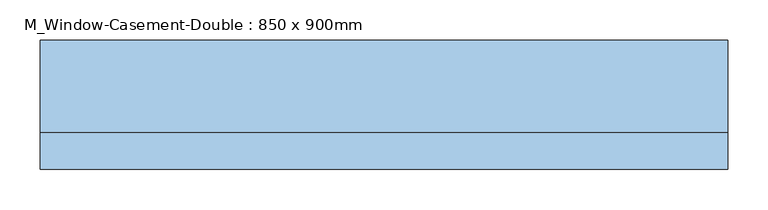
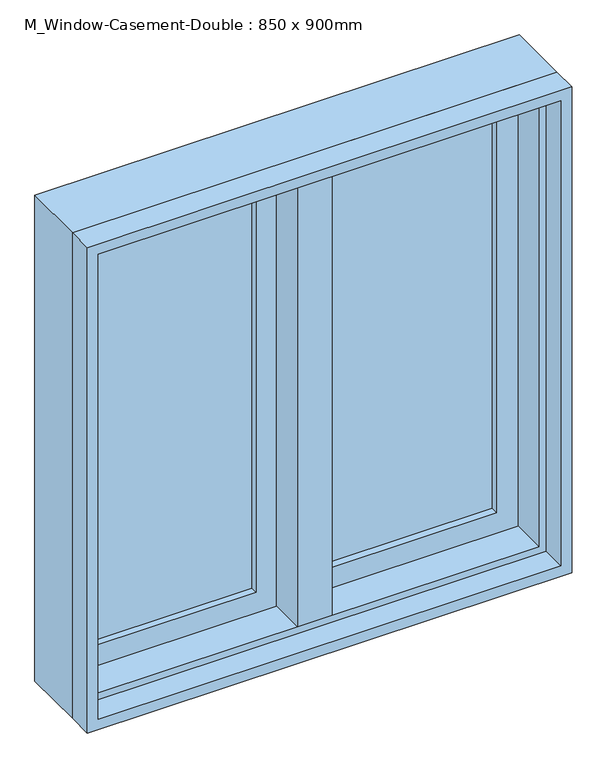
"""IFC4 building model written with IfcOpenShell, lengths in millimetres: window geometry, M_Window-Casement-Double : 850 x 900mm."""

from ifc_helpers import new_model, si_unit, frame, origin, place, context, project, spatial, polyline, outline, extrude, faceted_brep, source, transform, mapped, element, save


def m_window_casement_double_850_x_900mm_77c4388a(model_context):
    return source(origin(), model_context, "Body", "SolidModel", [
        faceted_brep([(9.525, 89.05, 1787.3), (-9.525, 89.05, 1787.3), (-9.525, 38.25, 1787.3), (9.525, 38.25, 1787.3), (9.525, 89.05, 912.7), (9.525, 38.25, 912.7), (-9.525, 38.25, 912.7), (-9.525, 89.05, 912.7), (-9.525, 38.25, 931.75), (-9.525, 38.25, 1768.25), (-30.1625, 38.25, 931.75), (-30.1625, 38.25, 1768.25), (-30.1625, -25.25, 931.75), (-30.1625, -25.25, 1768.25), (30.1625, -25.25, 931.75), (30.1625, -25.25, 1768.25), (30.1625, 38.25, 931.75), (30.1625, 38.25, 1768.25), (9.525, 38.25, 931.75), (9.525, 38.25, 1768.25)], [[[0, 1, 2, 3]], [[4, 5, 6, 7]], [[1, 0, 4, 7]], [[2, 1, 7, 6, 8, 9]], [[9, 8, 10, 11]], [[11, 10, 12, 13]], [[13, 12, 14, 15]], [[15, 14, 16, 17]], [[17, 16, 18, 19]], [[0, 3, 19, 18, 5, 4]], [[18, 8, 6, 5]], [[9, 19, 3, 2]], [[8, 18, 16, 14, 12, 10]], [[19, 9, 11, 13, 15, 17]]]),
        extrude(outline(polyline([(-66.675, 70.0), (-66.675, 63.65), (-355.15, 63.65), (-355.15, 70.0), (-66.675, 70.0)])), frame((0.0, 0.0, 969.85), z_axis=(0.0, 0.0, 1.0), x_axis=(1.0, 0.0, 0.0)), (0.0, 0.0, 1.0), 760.3),
        extrude(outline(polyline([(-355.15, 50.95), (-355.15, 57.3), (-66.675, 57.3), (-66.675, 50.95), (-355.15, 50.95)])), frame((0.0, 0.0, 969.85), z_axis=(0.0, 0.0, 1.0), x_axis=(1.0, 0.0, 0.0)), (0.0, 0.0, 1.0), 760.3),
        extrude(outline(polyline([(355.15, 70.0), (355.15, 63.65), (66.675, 63.65), (66.675, 70.0), (355.15, 70.0)])), frame((0.0, 0.0, 969.85), z_axis=(0.0, 0.0, 1.0), x_axis=(1.0, 0.0, 0.0)), (0.0, 0.0, 1.0), 760.3),
        extrude(outline(polyline([(66.675, 50.95), (66.675, 57.3), (355.15, 57.3), (355.15, 50.95), (66.675, 50.95)])), frame((0.0, 0.0, 969.85), z_axis=(0.0, 0.0, 1.0), x_axis=(1.0, 0.0, 0.0)), (0.0, 0.0, 1.0), 760.3),
        extrude(outline(polyline([(1787.3, -412.3), (912.7, -412.3), (912.7, -9.525), (1787.3, -9.525), (1787.3, -412.3)]), holes=[polyline([(1730.15, -66.675), (969.85, -66.675), (969.85, -355.15), (1730.15, -355.15), (1730.15, -66.675)])]), frame((0.0, 38.25, 0.0), z_axis=(0.0, 1.0, 0.0), x_axis=(0.0, 0.0, 1.0)), (0.0, 0.0, 1.0), 44.45),
        extrude(outline(polyline([(912.7, 412.3), (1787.3, 412.3), (1787.3, 9.525), (912.7, 9.525), (912.7, 412.3)]), holes=[polyline([(969.85, 66.675), (1730.15, 66.675), (1730.15, 355.15), (969.85, 355.15), (969.85, 66.675)])]), frame((0.0, 38.25, 0.0), z_axis=(0.0, 1.0, 0.0), x_axis=(0.0, 0.0, 1.0)), (0.0, 0.0, 1.0), 44.45),
        extrude(outline(polyline([(1800.0, -425.0), (900.0, -425.0), (900.0, 425.0), (1800.0, 425.0), (1800.0, -425.0)]), holes=[polyline([(1780.95, 405.95), (919.05, 405.95), (919.05, -405.95), (1780.95, -405.95), (1780.95, 405.95)])]), frame((0.0, -70.0, 0.0), z_axis=(0.0, 1.0, 0.0), x_axis=(0.0, 0.0, 1.0)), (0.0, 0.0, 1.0), 44.75),
        faceted_brep([(393.25, 38.25, 1768.25), (393.25, -25.25, 1768.25), (-393.25, -25.25, 1768.25), (-393.25, 38.25, 1768.25), (412.3, 89.05, 1787.3), (412.3, 38.25, 1787.3), (-412.3, 38.25, 1787.3), (-412.3, 89.05, 1787.3), (425.0, -25.25, 1800.0), (425.0, 89.05, 1800.0), (-425.0, 89.05, 1800.0), (-425.0, -25.25, 1800.0), (-393.25, -25.25, 931.75), (-393.25, 38.25, 931.75), (-412.3, 38.25, 912.7), (-412.3, 89.05, 912.7), (-425.0, 89.05, 900.0), (-425.0, -25.25, 900.0), (393.25, -25.25, 931.75), (393.25, 38.25, 931.75), (412.3, 38.25, 912.7), (412.3, 89.05, 912.7), (425.0, 89.05, 900.0), (425.0, -25.25, 900.0)], [[[0, 1, 2, 3]], [[4, 5, 6, 7]], [[8, 9, 10, 11]], [[3, 2, 12, 13]], [[7, 6, 14, 15]], [[11, 10, 16, 17]], [[13, 12, 18, 19]], [[15, 14, 20, 21]], [[17, 16, 22, 23]], [[11, 17, 23, 8], [1, 18, 12, 2]], [[19, 18, 1, 0]], [[5, 20, 14, 6], [3, 13, 19, 0]], [[21, 20, 5, 4]], [[23, 22, 9, 8]], [[9, 22, 16, 10], [7, 15, 21, 4]]]),
    ])


if __name__ == "__main__":
    model = new_model("IFC4")
    model_context = context("Model", 3, world=origin())
    ifc_project = project(units=[si_unit("LENGTHUNIT", "METRE", prefix="MILLI")], contexts=[model_context])
    site = spatial("IfcSite", under=ifc_project)
    building = spatial("IfcBuilding", under=site)
    placement = place(None, origin())
    m_window_casement_double_850_x_900mm_shape = m_window_casement_double_850_x_900mm_77c4388a(model_context)
    element("IfcWindow", 1, ObjectType="M_Window-Casement-Double : 850 x 900mm", at=placement, inside=building, context=model_context, shape_type="MappedRepresentation", body=[
        mapped(m_window_casement_double_850_x_900mm_shape, transform((0.0, 0.0, 0.0), x_axis=(1.0, 0.0, 0.0), y_axis=(0.0, 1.0, 0.0), z_axis=(0.0, 0.0, 1.0))),
    ])
    save(model, "model.ifc")

# Revit data of these elements
# Type "M_Window-Casement-Double : 850 x 900mm"
#   Type Mark = "23"
#   Fire Rating = "0.5h"
#   Assembly Code = "B2020100"
#   Analytic Construction = "Double glazing - domestic"
#   Frame Extension [instance default] = 0.020833 ft
#   Window Inset [instance default] = 0 ft
#   Wall Thickness [instance default] = 0.492126 ft
#   Interior Wall Closure [instance default] = 0.179626 ft
#   Half Width = 1.394357 ft
#   Visual Light Transmittance = 0.81
#   Thermal Resistance (R) = 0.319569 (m²·K)/W
#   Solar Heat Gain Coefficient = 0.76
#   Rough Width = 2.837927 ft
#   Rough Height = 3.001969 ft
#   Height = 2.952756 ft
#   Heat Transfer Coefficient (U) = 3.12929 W/(m²·K)
#   Exterior Wall Closure [instance default] = 0.104331 ft
#   Extension Jamb [instance default] = 0.179626 ft
#   Default Sill Height = 2.952756 ft
#   Width = 2.788714 ft
#   Define Thermal Properties by = 0
#   Muntin Visibility = yes
#   Interior Trim Visibility [instance default] = yes
#   Exterior Trim Visibility [instance default] = yes
#   Extension Jamb Visibility [instance default] = yes
#   Interior Trim Material = Wood - Stained
#   Muntin Pattern = M_Muntin Pattern_2x2 : M_Muntin Pattern_2x2
#   Interior Trim = M_Trim-Window-Interior-Flat : Picture Frame
#   Interior Frame Material = Wood - Stained
#   Glass Panel Material = Glass
#   Exterior Trim Material = Clad - White
#   Exterior Trim = M_Trim-Window-Exterior-Flat : with Sill
#   Exterior Frame Material = Clad - White
#   Wall Closure = (empty or 0)
# Element 1 (IfcWindow, "M_Window-Casement-Double : 850 x 900mm")
#   Wall Thickness = 0.459318 ft
#   Extension Jamb = 0.146818 ft
#   Materials on its faces: "Wood - Stained", "Glass", "Clad - White"
# Materials
#   "Wood - Stained": class "Wood", colour RGB 224 178 126, transparency 0, Cost = 0
#   "Glass": class "Glass", colour RGB 0 128 192, transparency 0.9, Description = "Soda Lime Glass", Cost = 0
#   "Clad - White": class "Wood", colour RGB 242 242 238, transparency 0, Cost = 0
